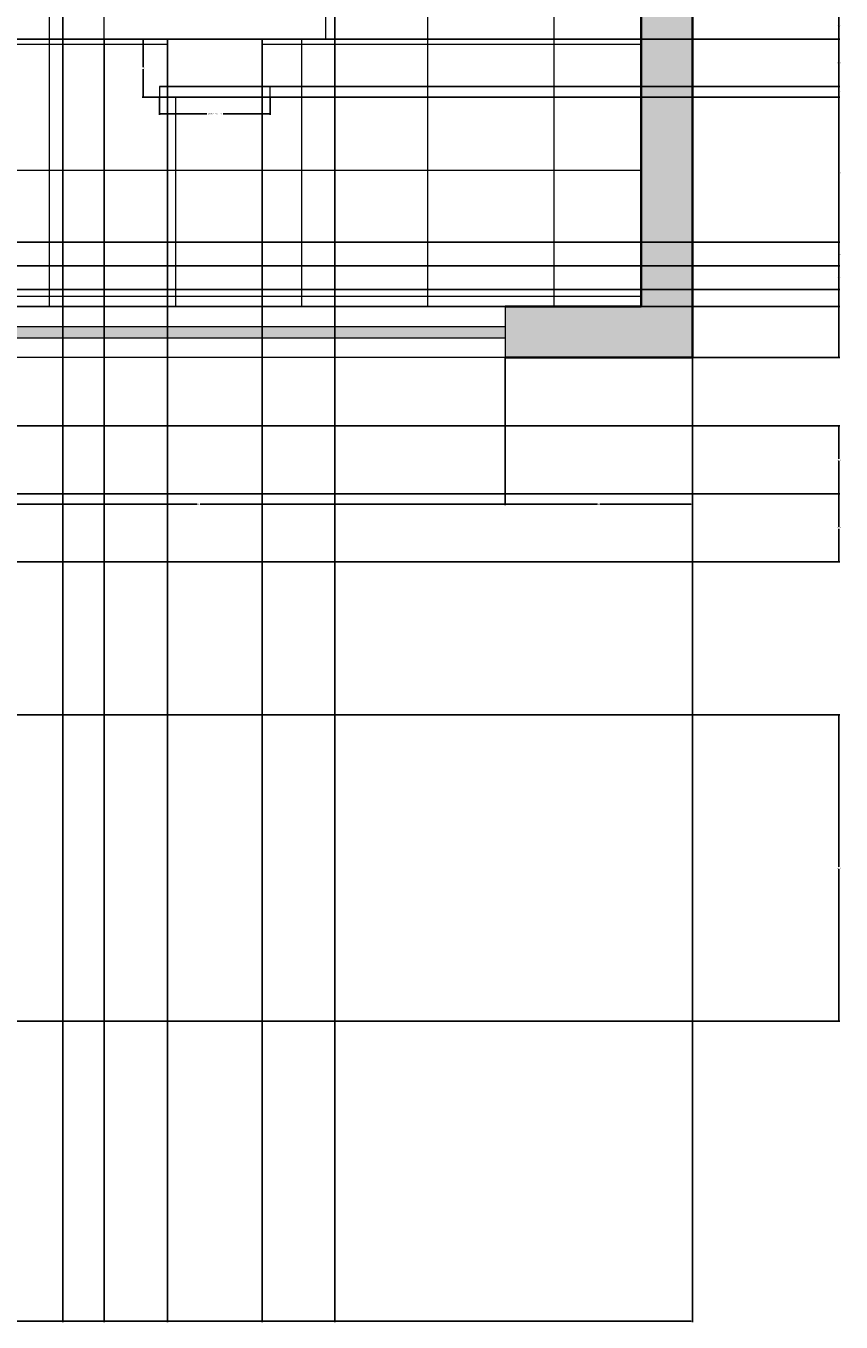
# Model space of a CAD drawing. Units: inches. Extents: x 6 to 575, y 34 to 566.
# Tile 14 of 21: x 431 to 575, y 34 to 262. Entities that reach past the tile are written whole.
import ezdxf

# ---------------------------------------------------------------- set-up
doc = ezdxf.new("R2010")
doc.units = ezdxf.units.IN
for name, color, linetype, lineweight in [('A-ANNO-DIMS', 2, 'Continuous', 18), ('A-FLOR-PATT', 252, 'Continuous', 9), ('A-GLAZ-PATT', 4, 'Continuous', 9), ('A-WALL-PATT', 251, 'Continuous', 9), ('FUR', 2, 'Continuous', 18), ('WALLS', 7, 'Continuous', 35), ('WINDOWS', 4, 'Continuous', 20)]:
    doc.layers.add(name, color=color, linetype=linetype, lineweight=lineweight)
doc.styles.get("Standard").update_dxf_attribs({"font": 'arial.ttf'})
doc.dimstyles.get("Standard").update_dxf_attribs({"dimtxt": 0.18, "dimasz": 0.18, "dimexe": 0.18, "dimexo": 0.0625, "dimgap": 0.09, "dimtad": 0, "dimtih": 1, "dimtoh": 1, "dimdec": 4, "dimzin": 0, "dimdsep": 46, "dimtxsty": 'Standard', "dimcen": 0.09, "dimadec": 0, "dimazin": 0, "dimtfac": 1, "dimtdec": 4, "dimtofl": 0, "dimtmove": 0, "dimatfit": 3, "dimfxl": 1, "dimtolj": 1, "dimtzin": 0, "dimarcsym": 0})

# ---------------------------------------------------------------- blocks, each defined once
blk = doc.blocks.new('CHAIR-DINING')
for points in [[(0, 1.4), (8.35, 1.4), (8.35, 0), (10.22, 0), (10.22, 19.51), (8.35, 19.51), (8.35, 18.1), (0, 18.1)], [(8.35, 18.1), (8.35, 1.4)]]:
    blk.add_lwpolyline(points)
blk = doc.blocks.new('*D11')
at = {"layer": 'A-ANNO-DIMS', "color": 0, "lineweight": -2, "transparency": 16777216}
for p, q in [((454.77, 249.64), (454.77, 246.59)), ((474.28, 249.64), (474.28, 246.59)), ((454.95, 246.77), (463.1, 246.77)), ((474.1, 246.77), (465.95, 246.77))]:
    blk.add_line(p, q, dxfattribs=at)
at = {"layer": 'A-ANNO-DIMS', "color": 0, "transparency": 16777216}
for points in [[(454.95, 246.8), (454.95, 246.74), (454.77, 246.77)], [(474.1, 246.8), (474.1, 246.74), (474.28, 246.77)]]:
    blk.add_solid(points, dxfattribs=at)
at = {"layer": 'Defpoints', "color": 0, "transparency": 16777216}
for p in [(454.77, 249.7), (474.28, 249.7), (474.28, 246.77)]:
    blk.add_point(p, dxfattribs=at)
at = {"layer": 'A-ANNO-DIMS', "color": 0, "transparency": 16777216, "insert": (464.53, 246.77), "char_height": 0.18, "attachment_point": 5}
blk.add_mtext('\\A1;DINING CHAIR 20 TYP.', dxfattribs=at)
blk = doc.blocks.new('*D12')
at = {"layer": 'A-ANNO-DIMS', "color": 0, "lineweight": -2, "transparency": 16777216}
for p, q in [((454.71, 259.92), (451.67, 259.92)), ((451.85, 259.74), (451.85, 254.99)), ((451.85, 249.88), (451.85, 254.63)), ((454.71, 249.7), (451.67, 249.7))]:
    blk.add_line(p, q, dxfattribs=at)
at = {"layer": 'A-ANNO-DIMS', "color": 0, "transparency": 16777216}
for points in [[(451.82, 259.74), (451.88, 259.74), (451.85, 259.92)], [(451.82, 249.88), (451.88, 249.88), (451.85, 249.7)]]:
    blk.add_solid(points, dxfattribs=at)
at = {"layer": 'Defpoints', "color": 0, "transparency": 16777216}
for p in [(454.77, 259.92), (451.85, 249.7), (454.77, 249.7)]:
    blk.add_point(p, dxfattribs=at)
at = {"layer": 'A-ANNO-DIMS', "color": 0, "transparency": 16777216, "insert": (451.85, 254.81), "char_height": 0.18, "attachment_point": 5}
blk.add_mtext('\\A1;10 TYP.', dxfattribs=at)
blk = doc.blocks.new('*D29')
at = {"layer": 'A-ANNO-DIMS', "color": 0, "lineweight": -2, "transparency": 16777216}
for p, q in [((32.66, 203.74), (32.66, 33.76)), ((548.66, 203.74), (548.66, 33.76)), ((32.84, 33.94), (290.37, 33.94)), ((548.48, 33.94), (290.95, 33.94))]:
    blk.add_line(p, q, dxfattribs=at)
at = {"layer": 'A-ANNO-DIMS', "color": 0, "transparency": 16777216}
for points in [[(32.84, 33.97), (32.84, 33.91), (32.66, 33.94)], [(548.48, 33.97), (548.48, 33.91), (548.66, 33.94)]]:
    blk.add_solid(points, dxfattribs=at)
at = {"layer": 'Defpoints', "color": 0, "transparency": 16777216}
for p in [(32.66, 203.8), (548.66, 203.8), (548.66, 33.94)]:
    blk.add_point(p, dxfattribs=at)
at = {"layer": 'A-ANNO-DIMS', "color": 0, "transparency": 16777216, "insert": (290.66, 33.94), "char_height": 0.18, "attachment_point": 5}
blk.add_mtext('\\A1;516', dxfattribs=at)
blk = doc.blocks.new('*D40')
at = {"layer": 'A-ANNO-DIMS', "color": 0, "lineweight": -2, "transparency": 16777216}
for p, q in [((407.66, 203.74), (407.66, 177.79)), ((515.66, 203.74), (515.66, 177.79)), ((407.84, 177.97), (461.38, 177.97)), ((515.48, 177.97), (461.94, 177.97))]:
    blk.add_line(p, q, dxfattribs=at)
at = {"layer": 'A-ANNO-DIMS', "color": 0, "transparency": 16777216}
for points in [[(407.84, 178), (407.84, 177.94), (407.66, 177.97)], [(515.48, 178), (515.48, 177.94), (515.66, 177.97)]]:
    blk.add_solid(points, dxfattribs=at)
at = {"layer": 'Defpoints', "color": 0, "transparency": 16777216}
for p in [(407.66, 203.8), (515.66, 203.8), (407.66, 177.97)]:
    blk.add_point(p, dxfattribs=at)
at = {"layer": 'A-ANNO-DIMS', "color": 0, "transparency": 16777216, "insert": (461.66, 177.97), "char_height": 0.18, "attachment_point": 5}
blk.add_mtext('\\A1;108', dxfattribs=at)
blk = doc.blocks.new('*D41')
at = {"layer": 'A-ANNO-DIMS', "color": 0, "lineweight": -2, "transparency": 16777216}
for p, q in [((515.66, 203.74), (515.66, 177.79)), ((548.66, 203.74), (548.66, 177.79)), ((515.84, 177.97), (531.94, 177.97)), ((548.48, 177.97), (532.38, 177.97))]:
    blk.add_line(p, q, dxfattribs=at)
at = {"layer": 'A-ANNO-DIMS', "color": 0, "transparency": 16777216}
for points in [[(515.84, 178), (515.84, 177.94), (515.66, 177.97)], [(548.48, 178), (548.48, 177.94), (548.66, 177.97)]]:
    blk.add_solid(points, dxfattribs=at)
at = {"layer": 'Defpoints', "color": 0, "transparency": 16777216}
for p in [(515.66, 203.8), (548.66, 203.8), (515.66, 177.97)]:
    blk.add_point(p, dxfattribs=at)
at = {"layer": 'A-ANNO-DIMS', "color": 0, "transparency": 16777216, "insert": (532.16, 177.97), "char_height": 0.18, "attachment_point": 5}
blk.add_mtext('\\A1;33', dxfattribs=at)
blk = doc.blocks.new('*D44')
at = {"layer": 'A-ANNO-DIMS', "color": 0, "lineweight": -2, "transparency": 16777216}
for p, q in [((548.72, 270.8), (574.68, 270.8)), ((574.5, 270.62), (574.5, 237.48)), ((574.5, 203.98), (574.5, 237.12)), ((548.72, 203.8), (574.68, 203.8))]:
    blk.add_line(p, q, dxfattribs=at)
at = {"layer": 'A-ANNO-DIMS', "color": 0, "transparency": 16777216}
for points in [[(574.47, 270.62), (574.53, 270.62), (574.5, 270.8)], [(574.47, 203.98), (574.53, 203.98), (574.5, 203.8)]]:
    blk.add_solid(points, dxfattribs=at)
at = {"layer": 'Defpoints', "color": 0, "transparency": 16777216}
for p in [(548.66, 270.8), (574.5, 270.8), (548.66, 203.8)]:
    blk.add_point(p, dxfattribs=at)
at = {"layer": 'A-ANNO-DIMS', "color": 0, "transparency": 16777216, "insert": (574.5, 237.3), "char_height": 0.18, "attachment_point": 5}
blk.add_mtext('\\A1;67', dxfattribs=at)
blk = doc.blocks.new('*D51')
at = {"layer": 'A-ANNO-DIMS', "color": 0, "lineweight": -2, "transparency": 16777216}
for p, q in [((437.69, 435.25), (437.69, 33.76)), ((485.67, 435.25), (485.67, 33.76)), ((437.87, 33.94), (461.28, 33.94)), ((485.49, 33.94), (462.08, 33.94))]:
    blk.add_line(p, q, dxfattribs=at)
at = {"layer": 'A-ANNO-DIMS', "color": 0, "transparency": 16777216}
for points in [[(437.87, 33.97), (437.87, 33.91), (437.69, 33.94)], [(485.49, 33.97), (485.49, 33.91), (485.67, 33.94)]]:
    blk.add_solid(points, dxfattribs=at)
at = {"layer": 'Defpoints', "color": 0, "transparency": 16777216}
for p in [(437.69, 435.31), (485.67, 435.31), (485.67, 33.94)]:
    blk.add_point(p, dxfattribs=at)
at = {"layer": 'A-ANNO-DIMS', "color": 0, "transparency": 16777216, "insert": (461.68, 33.94), "char_height": 0.18, "attachment_point": 5}
blk.add_mtext('\\A1;47.98', dxfattribs=at)
blk = doc.blocks.new('*D54')
at = {"layer": 'A-ANNO-DIMS', "color": 0, "lineweight": -2, "transparency": 16777216}
for p, q in [((444.96, 337.94), (6.65, 337.94)), ((6.83, 337.76), (6.83, 299.11)), ((6.83, 260.1), (6.83, 298.75)), ((444.96, 259.92), (6.65, 259.92))]:
    blk.add_line(p, q, dxfattribs=at)
at = {"layer": 'A-ANNO-DIMS', "color": 0, "transparency": 16777216}
for points in [[(6.8, 337.76), (6.86, 337.76), (6.83, 337.94)], [(6.8, 260.1), (6.86, 260.1), (6.83, 259.92)]]:
    blk.add_solid(points, dxfattribs=at)
at = {"layer": 'Defpoints', "color": 0, "transparency": 16777216}
for p in [(6.83, 337.94), (445.02, 337.94), (445.02, 259.92)]:
    blk.add_point(p, dxfattribs=at)
at = {"layer": 'A-ANNO-DIMS', "color": 0, "transparency": 16777216, "insert": (6.83, 298.93), "char_height": 0.18, "attachment_point": 5}
blk.add_mtext('\\A1;78.02', dxfattribs=at)
blk = doc.blocks.new('*D74')
at = {"layer": 'A-ANNO-DIMS', "color": 0, "lineweight": -2, "transparency": 16777216}
for p, q in [((384.14, 191.79), (574.68, 191.79)), ((574.5, 191.61), (574.5, 185.96)), ((574.5, 179.95), (574.5, 185.6)), ((384.14, 179.77), (574.68, 179.77))]:
    blk.add_line(p, q, dxfattribs=at)
at = {"layer": 'A-ANNO-DIMS', "color": 0, "transparency": 16777216}
for points in [[(574.47, 191.61), (574.53, 191.61), (574.5, 191.79)], [(574.47, 179.95), (574.53, 179.95), (574.5, 179.77)]]:
    blk.add_solid(points, dxfattribs=at)
at = {"layer": 'Defpoints', "color": 0, "transparency": 16777216}
for p in [(384.08, 191.79), (384.08, 179.77), (574.5, 179.77)]:
    blk.add_point(p, dxfattribs=at)
at = {"layer": 'A-ANNO-DIMS', "color": 0, "transparency": 16777216, "insert": (574.5, 185.78), "char_height": 0.18, "attachment_point": 5}
blk.add_mtext('\\A1;12.015', dxfattribs=at)
blk = doc.blocks.new('*D75')
at = {"layer": 'A-ANNO-DIMS', "color": 0, "lineweight": -2, "transparency": 16777216}
for p, q in [((384.14, 179.77), (574.68, 179.77)), ((574.5, 179.59), (574.5, 173.95)), ((574.5, 167.94), (574.5, 173.58)), ((384.14, 167.76), (574.68, 167.76))]:
    blk.add_line(p, q, dxfattribs=at)
at = {"layer": 'A-ANNO-DIMS', "color": 0, "transparency": 16777216}
for points in [[(574.47, 179.59), (574.53, 179.59), (574.5, 179.77)], [(574.47, 167.94), (574.53, 167.94), (574.5, 167.76)]]:
    blk.add_solid(points, dxfattribs=at)
at = {"layer": 'Defpoints', "color": 0, "transparency": 16777216}
for p in [(384.08, 179.77), (384.08, 167.76), (574.5, 167.76)]:
    blk.add_point(p, dxfattribs=at)
at = {"layer": 'A-ANNO-DIMS', "color": 0, "transparency": 16777216, "insert": (574.5, 173.76), "char_height": 0.18, "attachment_point": 5}
blk.add_mtext('\\A1;12.015', dxfattribs=at)
blk = doc.blocks.new('*D82')
at = {"layer": 'A-ANNO-DIMS', "color": 0, "lineweight": -2, "transparency": 16777216}
for p, q in [((338.25, 140.81), (574.68, 140.81)), ((574.5, 140.63), (574.5, 113.99)), ((574.5, 86.98), (574.5, 113.62)), ((338.25, 86.8), (574.68, 86.8))]:
    blk.add_line(p, q, dxfattribs=at)
at = {"layer": 'A-ANNO-DIMS', "color": 0, "transparency": 16777216}
for points in [[(574.47, 140.63), (574.53, 140.63), (574.5, 140.81)], [(574.47, 86.98), (574.53, 86.98), (574.5, 86.8)]]:
    blk.add_solid(points, dxfattribs=at)
at = {"layer": 'Defpoints', "color": 0, "transparency": 16777216}
for p in [(338.19, 140.81), (574.5, 140.81), (338.19, 86.8)]:
    blk.add_point(p, dxfattribs=at)
at = {"layer": 'A-ANNO-DIMS', "color": 0, "transparency": 16777216, "insert": (574.5, 113.81), "char_height": 0.18, "attachment_point": 5}
blk.add_mtext('\\A1;54.02', dxfattribs=at)
blk = doc.blocks.new('*D138')
at = {"layer": 'A-ANNO-DIMS', "color": 0, "lineweight": -2, "transparency": 16777216}
for p, q in [((445.02, 259.86), (445.02, 33.76)), ((383.66, 212.74), (383.66, 33.76)), ((383.84, 33.94), (413.95, 33.94)), ((444.84, 33.94), (414.73, 33.94))]:
    blk.add_line(p, q, dxfattribs=at)
at = {"layer": 'A-ANNO-DIMS', "color": 0, "transparency": 16777216}
for points in [[(383.84, 33.97), (383.84, 33.91), (383.66, 33.94)], [(444.84, 33.97), (444.84, 33.91), (445.02, 33.94)]]:
    blk.add_solid(points, dxfattribs=at)
at = {"layer": 'Defpoints', "color": 0, "transparency": 16777216}
for p in [(445.02, 259.92), (383.66, 212.8), (445.02, 33.94)]:
    blk.add_point(p, dxfattribs=at)
at = {"layer": 'A-ANNO-DIMS', "color": 0, "transparency": 16777216, "insert": (414.34, 33.94), "char_height": 0.18, "attachment_point": 5}
blk.add_mtext('\\A1;61.36', dxfattribs=at)
blk = doc.blocks.new('*D139')
at = {"layer": 'A-ANNO-DIMS', "color": 0, "lineweight": -2, "transparency": 16777216}
for p, q in [((445.08, 259.92), (574.68, 259.92)), ((574.5, 259.74), (574.5, 236.54)), ((574.5, 212.98), (574.5, 236.18)), ((383.72, 212.8), (574.68, 212.8))]:
    blk.add_line(p, q, dxfattribs=at)
at = {"layer": 'A-ANNO-DIMS', "color": 0, "transparency": 16777216}
for points in [[(574.47, 259.74), (574.53, 259.74), (574.5, 259.92)], [(574.47, 212.98), (574.53, 212.98), (574.5, 212.8)]]:
    blk.add_solid(points, dxfattribs=at)
at = {"layer": 'Defpoints', "color": 0, "transparency": 16777216}
for p in [(445.02, 259.92), (574.5, 259.92), (383.66, 212.8)]:
    blk.add_point(p, dxfattribs=at)
at = {"layer": 'A-ANNO-DIMS', "color": 0, "transparency": 16777216, "insert": (574.5, 236.36), "char_height": 0.18, "attachment_point": 5}
blk.add_mtext('\\A1;47.12', dxfattribs=at)
blk = doc.blocks.new('*D143')
at = {"layer": 'A-ANNO-DIMS', "color": 0, "lineweight": -2, "transparency": 16777216}
for p, q in [((456.24, 259.92), (574.68, 259.92)), ((574.5, 259.74), (574.5, 255.93)), ((574.5, 251.75), (574.5, 255.56)), ((454.84, 251.57), (574.68, 251.57))]:
    blk.add_line(p, q, dxfattribs=at)
at = {"layer": 'A-ANNO-DIMS', "color": 0, "transparency": 16777216}
for points in [[(574.47, 259.74), (574.53, 259.74), (574.5, 259.92)], [(574.47, 251.75), (574.53, 251.75), (574.5, 251.57)]]:
    blk.add_solid(points, dxfattribs=at)
at = {"layer": 'Defpoints', "color": 0, "transparency": 16777216}
for p in [(456.18, 259.92), (454.77, 251.57), (574.5, 251.57)]:
    blk.add_point(p, dxfattribs=at)
at = {"layer": 'A-ANNO-DIMS', "color": 0, "transparency": 16777216, "insert": (574.5, 255.75), "char_height": 0.18, "attachment_point": 5}
blk.add_mtext('\\A1;8.348', dxfattribs=at)
blk = doc.blocks.new('*D144')
at = {"layer": 'A-ANNO-DIMS', "color": 0, "lineweight": -2, "transparency": 16777216}
for p, q in [((456.18, 259.86), (456.18, 33.76)), ((472.87, 259.86), (472.87, 33.76)), ((456.36, 33.94), (464.07, 33.94)), ((472.69, 33.94), (464.98, 33.94))]:
    blk.add_line(p, q, dxfattribs=at)
at = {"layer": 'A-ANNO-DIMS', "color": 0, "transparency": 16777216}
for points in [[(456.36, 33.97), (456.36, 33.91), (456.18, 33.94)], [(472.69, 33.97), (472.69, 33.91), (472.87, 33.94)]]:
    blk.add_solid(points, dxfattribs=at)
at = {"layer": 'Defpoints', "color": 0, "transparency": 16777216}
for p in [(456.18, 259.92), (472.87, 259.92), (472.87, 33.94)]:
    blk.add_point(p, dxfattribs=at)
at = {"layer": 'A-ANNO-DIMS', "color": 0, "transparency": 16777216, "insert": (464.53, 33.94), "char_height": 0.18, "attachment_point": 5}
blk.add_mtext('\\A1;16.696', dxfattribs=at)
blk = doc.blocks.new('*D145')
at = {"layer": 'A-ANNO-DIMS', "color": 0, "lineweight": -2, "transparency": 16777216}
for p, q in [((454.84, 251.57), (574.68, 251.57)), ((574.5, 251.39), (574.5, 250.82)), ((454.84, 249.7), (574.68, 249.7)), ((574.5, 249.88), (574.5, 250.45))]:
    blk.add_line(p, q, dxfattribs=at)
at = {"layer": 'A-ANNO-DIMS', "color": 0, "transparency": 16777216}
for points in [[(574.47, 251.39), (574.53, 251.39), (574.5, 251.57)], [(574.47, 249.88), (574.53, 249.88), (574.5, 249.7)]]:
    blk.add_solid(points, dxfattribs=at)
at = {"layer": 'Defpoints', "color": 0, "transparency": 16777216}
for p in [(454.77, 251.57), (454.77, 249.7), (574.5, 249.7)]:
    blk.add_point(p, dxfattribs=at)
at = {"layer": 'A-ANNO-DIMS', "color": 0, "transparency": 16777216, "insert": (574.5, 250.64), "char_height": 0.18, "attachment_point": 5}
blk.add_mtext('\\A1;1.87', dxfattribs=at)
blk = doc.blocks.new('*D148')
at = {"layer": 'A-ANNO-DIMS', "color": 0, "lineweight": -2, "transparency": 16777216}
for p, q in [((494.31, 264.6), (574.68, 264.6)), ((574.5, 264.42), (574.5, 262.44)), ((574.5, 260.1), (574.5, 262.08)), ((484.09, 259.92), (574.68, 259.92))]:
    blk.add_line(p, q, dxfattribs=at)
at = {"layer": 'A-ANNO-DIMS', "color": 0, "transparency": 16777216}
for points in [[(574.47, 264.42), (574.53, 264.42), (574.5, 264.6)], [(574.47, 260.1), (574.53, 260.1), (574.5, 259.92)]]:
    blk.add_solid(points, dxfattribs=at)
at = {"layer": 'Defpoints', "color": 0, "transparency": 16777216}
for p in [(494.25, 264.6), (574.5, 264.6), (484.03, 259.92)]:
    blk.add_point(p, dxfattribs=at)
at = {"layer": 'A-ANNO-DIMS', "color": 0, "transparency": 16777216, "insert": (574.5, 262.26), "char_height": 0.18, "attachment_point": 5}
blk.add_mtext('\\A1;4.681', dxfattribs=at)
blk = doc.blocks.new('*D149')
at = {"layer": 'A-ANNO-DIMS', "color": 0, "lineweight": -2, "transparency": 16777216}
for p, q in [((445.02, 259.86), (445.02, 33.76)), ((456.18, 259.86), (456.18, 33.76)), ((445.2, 33.94), (450.14, 33.94)), ((456, 33.94), (451.05, 33.94))]:
    blk.add_line(p, q, dxfattribs=at)
at = {"layer": 'A-ANNO-DIMS', "color": 0, "transparency": 16777216}
for points in [[(445.2, 33.97), (445.2, 33.91), (445.02, 33.94)], [(456, 33.97), (456, 33.91), (456.18, 33.94)]]:
    blk.add_solid(points, dxfattribs=at)
at = {"layer": 'Defpoints', "color": 0, "transparency": 16777216}
for p in [(445.02, 259.92), (456.18, 259.92), (456.18, 33.94)]:
    blk.add_point(p, dxfattribs=at)
at = {"layer": 'A-ANNO-DIMS', "color": 0, "transparency": 16777216, "insert": (450.6, 33.94), "char_height": 0.18, "attachment_point": 5}
blk.add_mtext('\\A1;11.157', dxfattribs=at)
blk = doc.blocks.new('*D212')
at = {"layer": 'A-ANNO-DIMS', "color": 0, "lineweight": -2, "transparency": 16777216}
for p, q in [((316.72, 219.96), (574.68, 219.96)), ((574.5, 219.78), (574.5, 218.06)), ((574.5, 215.98), (574.5, 217.7)), ((316.72, 215.8), (574.68, 215.8))]:
    blk.add_line(p, q, dxfattribs=at)
at = {"layer": 'A-ANNO-DIMS', "color": 0, "transparency": 16777216}
for points in [[(574.47, 219.78), (574.53, 219.78), (574.5, 219.96)], [(574.47, 215.98), (574.53, 215.98), (574.5, 215.8)]]:
    blk.add_solid(points, dxfattribs=at)
at = {"layer": 'Defpoints', "color": 0, "transparency": 16777216}
for p in [(316.66, 219.96), (574.5, 219.96), (316.66, 215.8)]:
    blk.add_point(p, dxfattribs=at)
at = {"layer": 'A-ANNO-DIMS', "color": 0, "transparency": 16777216, "insert": (574.5, 217.88), "char_height": 0.18, "attachment_point": 5}
blk.add_mtext('\\A1;4.16', dxfattribs=at)
blk = doc.blocks.new('*D216')
at = {"layer": 'A-ANNO-DIMS', "color": 0, "lineweight": -2, "transparency": 16777216}
for p, q in [((315.68, 224.12), (574.68, 224.12)), ((574.5, 223.94), (574.5, 222.22)), ((574.5, 220.14), (574.5, 221.86)), ((315.68, 219.96), (574.68, 219.96))]:
    blk.add_line(p, q, dxfattribs=at)
at = {"layer": 'A-ANNO-DIMS', "color": 0, "transparency": 16777216}
for points in [[(574.47, 223.94), (574.53, 223.94), (574.5, 224.12)], [(574.47, 220.14), (574.53, 220.14), (574.5, 219.96)]]:
    blk.add_solid(points, dxfattribs=at)
at = {"layer": 'Defpoints', "color": 0, "transparency": 16777216}
for p in [(315.62, 224.12), (574.5, 224.12), (315.62, 219.96)]:
    blk.add_point(p, dxfattribs=at)
at = {"layer": 'A-ANNO-DIMS', "color": 0, "transparency": 16777216, "insert": (574.5, 222.04), "char_height": 0.18, "attachment_point": 5}
blk.add_mtext('\\A1;4.16', dxfattribs=at)

msp = doc.modelspace()

# ---------------------------------------------------------------- hatches: boundary and pattern name
at = {"layer": 'A-FLOR-PATT'}
h = msp.add_hatch(dxfattribs=at)
h.set_pattern_fill('NET', color=256, scale=7)
h.set_pattern_definition([(0, (-98.035, 170.147), (0, 22.225), []), (90, (-98.035, 170.147), (-22.225, 1e-15), [])])
h.paths.add_polyline_path([(539.6586, 366.801), (539.6586, 378.801), (433.708, 378.801), (383.6586, 378.801), (383.6586, 278.801), (383.6586, 224.801), (383.6586, 212.801), (407.6586, 212.801), (515.6586, 212.801), (539.6586, 212.801), (539.6586, 270.801)])
h.paths.add_polyline_path([(434.8003, 333.3365), (436.6727, 333.3365), (436.6727, 331.9322), (445.0208, 331.9322), (445.0208, 337.9397), (456.1776, 337.9397), (456.1776, 346.2878), (454.7733, 346.2878), (454.7733, 348.1603), (474.2782, 348.1603), (474.2782, 346.2878), (472.8738, 346.2878), (472.8738, 337.9397), (484.0307, 337.9397), (484.0307, 331.9322), (492.3788, 331.9322), (492.3788, 333.3365), (494.2512, 333.3365), (494.2512, 313.8316), (492.3788, 313.8316), (492.3788, 315.158), (484.0307, 315.158), (484.0307, 307.278), (492.3788, 307.278), (492.3788, 308.6823), (494.2512, 308.6823), (494.2512, 289.1774), (492.3788, 289.1774), (492.3788, 290.5818), (484.0307, 290.5818), (484.0307, 282.7018), (492.3788, 282.7018), (492.3788, 284.1062), (494.2512, 284.1062), (494.2512, 264.6013), (492.3788, 264.6013), (492.3788, 266.0056), (484.0307, 266.0056), (484.0307, 259.9201), (472.8738, 259.9201), (472.8738, 251.572), (474.2782, 251.572), (474.2782, 249.6995), (454.7733, 249.6995), (454.7733, 251.572), (456.1776, 251.572), (456.1776, 259.9201), (445.0208, 259.9201), (445.0208, 266.0056), (436.6727, 266.0056), (436.6727, 264.6013), (434.8003, 264.6013), (434.8003, 284.1062), (436.6727, 284.1062), (436.6727, 282.7018), (445.0208, 282.7018), (445.0208, 290.5818), (436.6727, 290.5818), (436.6727, 289.1774), (434.8003, 289.1774), (434.8003, 308.6823), (436.6727, 308.6823), (436.6727, 307.278), (445.0208, 307.278), (445.0208, 315.158), (436.6727, 315.158), (436.6727, 313.8316), (434.8003, 313.8316)], flags=16)
h.paths.add_polyline_path([(532.9619, 436.5144), (533.9192, 437.0672), (533.9307, 437.0472, -0.12106636), (546.2274, 440.0689), (539.6586, 440.801), (539.6586, 450.6781), (515.7066, 450.6781), (515.7066, 507.3203), (407.6494, 507.3203), (407.6494, 449.3517), (383.6586, 449.3517), (383.6586, 382.801), (433.708, 382.801), (433.708, 406.831), (539.6586, 406.831), (539.6586, 412.801), (545.7108, 412.801), (545.7108, 414.4327)])
h.paths.add_polyline_path([(437.687, 435.3082), (437.687, 471.3533), (485.6691, 471.3533), (485.6691, 435.3082)], flags=16)
at = {"layer": 'A-GLAZ-PATT'}
h = msp.add_hatch(color=256, dxfattribs=at)
h.dxf.hatch_style = 1
h.paths.add_polyline_path([(36.1586, 224.801), (38.1586, 224.801), (38.1586, 272.801), (36.1586, 272.801)])
h.paths.add_polyline_path([(167.6586, 207.301), (167.6586, 209.301), (71.6586, 209.301), (71.6586, 207.301)])
h.paths.add_polyline_path([(264.6586, 219.301), (264.6586, 221.301), (246.6586, 221.301), (246.6586, 219.301)])
h.paths.add_polyline_path([(316.6586, 221.301), (316.6586, 219.301), (334.6586, 219.301), (334.6586, 221.301)])
h.paths.add_polyline_path([(515.6586, 207.301), (515.6586, 209.301), (407.6586, 209.301), (407.6586, 207.301)])
h.paths.add_polyline_path([(543.1586, 270.801), (545.1586, 270.801), (545.1586, 366.801), (543.1586, 366.801)])
h.paths.add_polyline_path([(407.9436, 536.301), (407.9436, 534.301), (455.9436, 534.301), (455.9436, 536.301)])
h.paths.add_polyline_path([(272.6586, 536.301), (272.6586, 534.301), (320.6586, 534.301), (320.6586, 536.301)])
at = {"layer": 'A-WALL-PATT'}
h = msp.add_hatch(color=256, dxfattribs=at)
h.dxf.hatch_style = 1
h.paths.add_polyline_path([(160.6586, 539.801), (32.6586, 539.801), (32.6586, 272.801), (41.6586, 272.801), (41.6586, 286.0643), (41.6586, 358.0764), (41.6586, 379.0637), (41.6586, 407.7709), (41.6194, 407.7709), (41.6194, 431.801), (82.8918, 431.801), (82.8918, 440.801), (65.6494, 440.801), (65.6494, 440.7732), (41.6194, 440.7732), (41.6194, 515.5941), (41.6586, 530.801), (117.6586, 530.801), (117.6586, 474.801), (120.6068, 474.801), (121.6586, 474.801), (121.6586, 530.801), (137.4275, 530.801), (137.4275, 530.8356), (141.2505, 530.8356), (160.6586, 530.801)])
h.paths.add_polyline_path([(71.6586, 212.801), (41.6586, 212.801), (41.6586, 224.801), (32.6586, 224.801), (32.6586, 203.801), (71.6586, 203.801)])
h.paths.add_polyline_path([(206.6586, 215.801), (246.6586, 215.801), (246.6586, 224.801), (206.6586, 224.801), (206.6586, 230.801), (201.8157, 230.801), (197.6586, 230.801), (197.6586, 212.801), (167.6586, 212.801), (167.6586, 203.801), (206.6586, 203.801)])
h.paths.add_polyline_path([(383.6586, 224.801), (334.6586, 224.801), (334.6586, 215.801), (374.6586, 215.801), (374.6586, 203.801), (384.0753, 203.801), (407.6586, 203.801), (407.6586, 212.801), (383.6586, 212.801)])
h.paths.add_polyline_path([(548.6586, 270.801), (539.6586, 270.801), (539.6586, 212.801), (515.6586, 212.801), (515.6586, 203.801), (548.6586, 203.801)])
h.paths.add_polyline_path([(548.6586, 412.801), (545.7108, 412.801), (539.6586, 412.801), (539.6586, 382.801), (433.708, 382.801), (433.708, 378.801), (539.6586, 378.801), (539.6586, 366.801), (548.6586, 366.801)])
h.paths.add_polyline_path([(548.6586, 539.801), (455.9436, 539.801), (455.9436, 530.801), (539.6586, 530.801), (539.6586, 440.801), (548.6586, 440.801)])
h.paths.add_polyline_path([(407.9436, 539.801), (362.6586, 539.801), (362.6586, 530.801), (374.6586, 530.801), (374.6586, 452.801), (354.6586, 452.801), (354.6586, 448.801), (374.6586, 448.801), (374.6586, 278.801), (383.6586, 278.801), (383.6586, 530.801), (407.9436, 530.801)])
h.paths.add_polyline_path([(338.6586, 539.801), (320.6586, 539.801), (320.6586, 530.801), (322.6586, 530.801), (322.6586, 448.801), (326.6586, 448.801), (326.6586, 530.801), (338.6586, 530.801)])
h.paths.add_polyline_path([(272.6586, 539.801), (184.6586, 539.801), (184.6586, 530.801), (197.6586, 530.801), (197.6586, 440.801), (176.6714, 440.801), (121.6586, 440.801), (121.6586, 446.801), (117.6586, 446.801), (117.6586, 440.801), (111.6586, 440.801), (111.6586, 431.801), (197.6586, 431.801), (197.6586, 407.7709), (197.6586, 276.801), (206.6586, 276.801), (206.6586, 530.801), (272.6586, 530.801)])

# ---------------------------------------------------------------- linework, layer by layer
at = {"layer": 'FUR'}
msp.add_lwpolyline([(484.0307, 337.9397), (484.0307, 259.9201), (445.0208, 259.9201), (445.0208, 337.9397)], close=True, dxfattribs=at)
at = {"layer": 'WALLS'}
for p, q in [((539.6586, 270.801), (539.6586, 212.801)), ((548.6586, 270.801), (548.6586, 203.801)), ((539.6586, 212.801), (515.6586, 212.801)), ((548.6586, 203.801), (515.6586, 203.801))]:
    msp.add_line(p, q, dxfattribs=at)
at = {"layer": 'WINDOWS'}
for p, q in [((515.6586, 212.801), (515.6586, 203.801)), ((407.6586, 209.301), (515.6586, 209.301)), ((407.6586, 207.301), (515.6586, 207.301))]:
    msp.add_line(p, q, dxfattribs=at)
msp.add_lwpolyline([(407.6586, 212.801), (515.6586, 212.801), (515.6586, 203.801), (407.6586, 203.801)], close=True, dxfattribs=at)

# ---------------------------------------------------------------- block references
at = {"layer": 'FUR', "rotation": 269.9999999999998}
msp.add_blockref('CHAIR-DINING', (454.7729, 259.9197), dxfattribs=at)

# ---------------------------------------------------------------- dimensions: what is measured, and where the dimension line sits
at = {"layer": 'A-ANNO-DIMS'}
for base, p1, p2, override, picture, middle in [((485.6691, 33.9447), (437.687, 435.3082), (485.6691, 435.3082), {"dimdec": 2, "dimlfac": 1, "dimrnd": 0, "dimzin": 0, "dimdsep": 46, "dimlunit": 2}, '*D51', (461.678, 33.9447)), ((445.0208, 33.9447), (383.6586, 212.801), (445.0208, 259.9201), {"dimdec": 2, "dimlfac": 1, "dimrnd": 0, "dimzin": 0, "dimdsep": 46, "dimlunit": 2}, '*D138', (414.3397, 33.9447)), ((456.1776, 33.9447), (445.0208, 259.9201), (456.1776, 259.9201), {"dimdec": 3, "dimlfac": 1, "dimrnd": 0, "dimzin": 0, "dimdsep": 46, "dimlunit": 2}, '*D149', (450.5992, 33.9447)), ((472.8738, 33.9447), (456.1776, 259.9201), (472.8738, 259.9201), {"dimdec": 3, "dimlfac": 1, "dimrnd": 0, "dimzin": 0, "dimdsep": 46, "dimlunit": 2}, '*D144', (464.5257, 33.9447)), ((548.6586, 33.9447), (32.6586, 203.801), (548.6586, 203.801), {"dimdec": 0, "dimlfac": 1, "dimrnd": 0, "dimzin": 0, "dimdsep": 46, "dimlunit": 2}, '*D29', (290.6586, 33.9447))]:
    dim = msp.add_linear_dim(base=base, p1=p1, p2=p2, dimstyle='Standard', override=override, dxfattribs=at)
    dim.commit()
    dim.dimension.update_dxf_attribs({"geometry": picture, "text_midpoint": middle})
for base, p1, p2, angle, override, picture, middle in [((6.8286, 337.9397), (445.0208, 259.9201), (445.0208, 337.9397), 90, {"dimdec": 2, "dimlfac": 1, "dimrnd": 0, "dimzin": 0, "dimdsep": 46, "dimlunit": 2}, '*D54', (6.8286, 298.9299)), ((574.4958, 270.801), (548.6586, 203.801), (548.6586, 270.801), 90, {"dimdec": 0, "dimlfac": 1, "dimrnd": 0, "dimzin": 0, "dimdsep": 46, "dimlunit": 2}, '*D44', (574.4958, 237.301)), ((574.4958, 264.6013), (484.0307, 259.9201), (494.2512, 264.6013), 90, {"dimdec": 3, "dimlfac": 1, "dimrnd": 0, "dimzin": 0, "dimdsep": 46, "dimlunit": 2}, '*D148', (574.4958, 262.2607)), ((574.4958, 259.9201), (383.6586, 212.801), (445.0208, 259.9201), 90, {"dimdec": 2, "dimlfac": 1, "dimrnd": 0, "dimzin": 0, "dimdsep": 46, "dimlunit": 2}, '*D139', (574.4958, 236.3605)), ((574.4958, 251.572), (456.1776, 259.9201), (454.7733, 251.572), 90, {"dimdec": 3, "dimlfac": 1, "dimrnd": 0, "dimzin": 0, "dimdsep": 46, "dimlunit": 2}, '*D143', (574.4958, 255.746)), ((574.4958, 249.6995), (454.7733, 251.572), (454.7733, 249.6995), 90, {"dimdec": 2, "dimlfac": 1, "dimrnd": 0, "dimzin": 0, "dimdsep": 46, "dimlunit": 2}, '*D145', (574.4958, 250.6357)), ((574.4958, 224.121), (315.6186, 219.961), (315.6186, 224.121), 90, {"dimdec": 2, "dimlfac": 1, "dimrnd": 0, "dimzin": 0, "dimdsep": 46, "dimlunit": 2}, '*D216', (574.4958, 222.041)), ((574.4958, 219.961), (316.6586, 215.801), (316.6586, 219.961), 90, {"dimdec": 2, "dimlfac": 1, "dimrnd": 0, "dimzin": 0, "dimdsep": 46, "dimlunit": 2}, '*D212', (574.4958, 217.881)), ((407.6586, 177.971), (515.6586, 203.801), (407.6586, 203.801), 180, {"dimdec": 0, "dimlfac": 1, "dimrnd": 0, "dimzin": 0, "dimdsep": 46, "dimlunit": 2}, '*D40', (461.6586, 177.971)), ((515.6586, 177.971), (548.6586, 203.801), (515.6586, 203.801), 180, {"dimdec": 0, "dimlfac": 1, "dimrnd": 0, "dimzin": 0, "dimdsep": 46, "dimlunit": 2}, '*D41', (532.1586, 177.971)), ((574.4958, 179.7709), (384.0753, 191.786), (384.0753, 179.7709), 90, {"dimdec": 3, "dimlfac": 1, "dimrnd": 0, "dimzin": 0, "dimdsep": 46, "dimlunit": 2}, '*D74', (574.4958, 185.7785)), ((574.4958, 167.7559), (384.0753, 179.7709), (384.0753, 167.7559), 90, {"dimdec": 3, "dimlfac": 1, "dimrnd": 0, "dimzin": 0, "dimdsep": 46, "dimlunit": 2}, '*D75', (574.4958, 173.7634)), ((574.4958, 140.8149), (338.1907, 86.7958), (338.1907, 140.8149), 90, {"dimdec": 2, "dimlfac": 1, "dimrnd": 0, "dimzin": 0, "dimdsep": 46, "dimlunit": 2}, '*D82', (574.4958, 113.8053))]:
    dim = msp.add_linear_dim(base=base, p1=p1, p2=p2, angle=angle, dimstyle='Standard', override=override, dxfattribs=at)
    dim.commit()
    dim.dimension.update_dxf_attribs({"geometry": picture, "text_midpoint": middle})
dim = msp.add_linear_dim(base=(451.8476, 249.6995), p1=(454.7733, 259.9201), p2=(454.7733, 249.6995), angle=270, text='<> TYP.', dimstyle='Standard', override={"dimdec": 0, "dimlfac": 1, "dimrnd": 0, "dimzin": 0, "dimdsep": 46, "dimlunit": 2}, dxfattribs=at)
dim.commit()
dim.dimension.update_dxf_attribs({"geometry": '*D12', "text_midpoint": (451.8476, 254.8098)})
dim = msp.add_linear_dim(base=(474.2782, 246.7738), p1=(454.7733, 249.6995), p2=(474.2782, 249.6995), text='DINING CHAIR <> TYP.', dimstyle='Standard', override={"dimdec": 0, "dimlfac": 1, "dimrnd": 0, "dimzin": 0, "dimdsep": 46, "dimlunit": 2}, dxfattribs=at)
dim.commit()
dim.dimension.update_dxf_attribs({"geometry": '*D11', "text_midpoint": (464.5257, 246.7738)})

doc.saveas('drawing.dxf')
